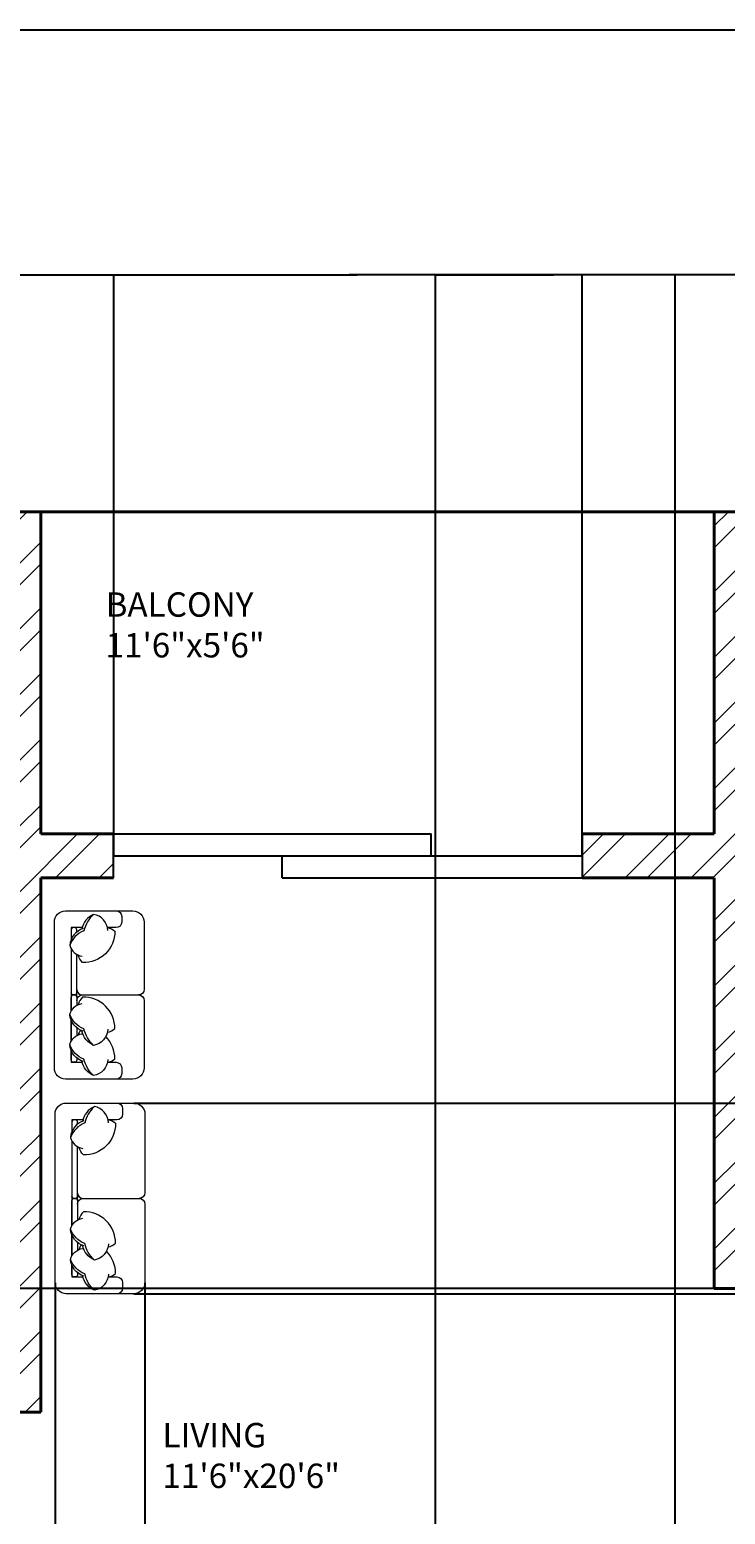
# Model space of a CAD drawing. Units: inches. Extents: x 1601 to 2297, y 1496 to 2631.
# Tile 51 of 57: x 1891 to 2033, y 2327 to 2631. Entities that reach past the tile are written whole.
import ezdxf

# ---------------------------------------------------------------- set-up
doc = ezdxf.new("R2010")
doc.units = ezdxf.units.IN
for name, color, linetype, lineweight in [('A-ANNO-DIMS', 2, 'Continuous', 18), ('A-ANNO-TTLB', 7, 'Continuous', 25), ('A-AREA-IDEN', 7, 'Continuous', 18), ('A-DOOR', 21, 'Continuous', 25), ('A-FURN', 8, 'Continuous', 18), ('A-WALL', 7, 'Continuous', 40), ('A-WALL-PATT', 215, 'Continuous', 13)]:
    doc.layers.add(name, color=color, linetype=linetype, lineweight=lineweight)
doc.styles.get("Standard").update_dxf_attribs({"font": 'arial.ttf'})
doc.dimstyles.get("Standard").update_dxf_attribs({"dimtxt": 0.18, "dimasz": 0.18, "dimexe": 0.18, "dimexo": 0.0625, "dimgap": 0.09, "dimtad": 0, "dimtih": 1, "dimtoh": 1, "dimdec": 4, "dimzin": 0, "dimdsep": 46, "dimtxsty": 'Standard', "dimcen": 0.09, "dimadec": 0, "dimazin": 0, "dimtfac": 1, "dimtdec": 4, "dimtofl": 0, "dimtmove": 0, "dimatfit": 3, "dimfxl": 1, "dimtolj": 1, "dimtzin": 0, "dimarcsym": 0})

# ---------------------------------------------------------------- blocks, each defined once
blk = doc.blocks.new('*D28')
at = {"layer": 'A-ANNO-DIMS', "color": 0, "lineweight": -2, "transparency": 16777216}
for p, q in [((1686.04, 2532.39), (1686.04, 2581.06)), ((1686.22, 2580.88), (1957.89, 2580.88)), ((2230.36, 2580.88), (1958.68, 2580.88)), ((2230.54, 2532.39), (2230.54, 2581.06))]:
    blk.add_line(p, q, dxfattribs=at)
at = {"layer": 'A-ANNO-DIMS', "color": 0, "transparency": 16777216}
for points in [[(1686.22, 2580.91), (1686.22, 2580.85), (1686.04, 2580.88)], [(2230.36, 2580.91), (2230.36, 2580.85), (2230.54, 2580.88)]]:
    blk.add_solid(points, dxfattribs=at)
at = {"layer": 'Defpoints', "color": 0, "transparency": 16777216}
for p in [(2230.54, 2580.88), (1686.04, 2532.33), (2230.54, 2532.33)]:
    blk.add_point(p, dxfattribs=at)
at = {"layer": 'A-ANNO-DIMS', "color": 0, "transparency": 16777216, "insert": (1958.29, 2580.88), "char_height": 0.18, "attachment_point": 5}
blk.add_mtext('\\A1;544.5', dxfattribs=at)
blk = doc.blocks.new('*D47')
at = {"layer": 'A-ANNO-DIMS', "color": 0, "lineweight": -2, "transparency": 16777216}
for p, q in [((1973.94, 2211.39), (1973.94, 2581.06)), ((1974.12, 2580.88), (1998.07, 2580.88)), ((2022.83, 2580.88), (1998.87, 2580.88)), ((2023.01, 2211.39), (2023.01, 2581.06))]:
    blk.add_line(p, q, dxfattribs=at)
at = {"layer": 'A-ANNO-DIMS', "color": 0, "transparency": 16777216}
for points in [[(1974.12, 2580.91), (1974.12, 2580.85), (1973.94, 2580.88)], [(2022.83, 2580.91), (2022.83, 2580.85), (2023.01, 2580.88)]]:
    blk.add_solid(points, dxfattribs=at)
at = {"layer": 'Defpoints', "color": 0, "transparency": 16777216}
for p in [(2023.01, 2580.88), (1973.94, 2211.33), (2023.01, 2211.33)]:
    blk.add_point(p, dxfattribs=at)
at = {"layer": 'A-ANNO-DIMS', "color": 0, "transparency": 16777216, "insert": (1998.47, 2580.88), "char_height": 0.18, "attachment_point": 5}
blk.add_mtext('\\A1;49.07', dxfattribs=at)
blk = doc.blocks.new('*D48')
at = {"layer": 'A-ANNO-DIMS', "color": 0, "lineweight": -2, "transparency": 16777216}
for p, q in [((2030.97, 2373.19), (1637.31, 2373.19)), ((1637.49, 2373.01), (1637.49, 2336.69)), ((1637.49, 2300.01), (1637.49, 2336.33)), ((2030.97, 2299.83), (1637.31, 2299.83))]:
    blk.add_line(p, q, dxfattribs=at)
at = {"layer": 'A-ANNO-DIMS', "color": 0, "transparency": 16777216}
for points in [[(1637.46, 2373.01), (1637.52, 2373.01), (1637.49, 2373.19)], [(1637.46, 2300.01), (1637.52, 2300.01), (1637.49, 2299.83)]]:
    blk.add_solid(points, dxfattribs=at)
at = {"layer": 'Defpoints', "color": 0, "transparency": 16777216}
for p in [(1637.49, 2373.19), (2031.04, 2373.19), (2031.04, 2299.83)]:
    blk.add_point(p, dxfattribs=at)
at = {"layer": 'A-ANNO-DIMS', "color": 0, "transparency": 16777216, "insert": (1637.49, 2336.51), "char_height": 0.18, "attachment_point": 5}
blk.add_mtext('\\A1;73.37', dxfattribs=at)
blk = doc.blocks.new('*D49')
at = {"layer": 'A-ANNO-DIMS', "color": 0, "lineweight": -2, "transparency": 16777216}
for p, q in [((1907.99, 2466.39), (1907.99, 2581.06)), ((1908.17, 2580.88), (1955.77, 2580.88)), ((2003.81, 2580.88), (1956.21, 2580.88)), ((2003.99, 2466.39), (2003.99, 2581.06))]:
    blk.add_line(p, q, dxfattribs=at)
at = {"layer": 'A-ANNO-DIMS', "color": 0, "transparency": 16777216}
for points in [[(1908.17, 2580.91), (1908.17, 2580.85), (1907.99, 2580.88)], [(2003.81, 2580.91), (2003.81, 2580.85), (2003.99, 2580.88)]]:
    blk.add_solid(points, dxfattribs=at)
at = {"layer": 'Defpoints', "color": 0, "transparency": 16777216}
for p in [(2003.99, 2580.88), (1907.99, 2466.33), (2003.99, 2466.33)]:
    blk.add_point(p, dxfattribs=at)
at = {"layer": 'A-ANNO-DIMS', "color": 0, "transparency": 16777216, "insert": (1955.99, 2580.88), "char_height": 0.18, "attachment_point": 5}
blk.add_mtext('\\A1;96', dxfattribs=at)
blk = doc.blocks.new('*D50')
at = {"layer": 'A-ANNO-DIMS', "color": 0, "lineweight": -2, "transparency": 16777216}
for p, q in [((1895.99, 2374.33), (1895.99, 1513.75)), ((1914.39, 2374.33), (1914.39, 1513.75)), ((1896.17, 1513.93), (1904.87, 1513.93)), ((1914.21, 1513.93), (1905.5, 1513.93))]:
    blk.add_line(p, q, dxfattribs=at)
at = {"layer": 'A-ANNO-DIMS', "color": 0, "transparency": 16777216}
for points in [[(1896.17, 1513.96), (1896.17, 1513.9), (1895.99, 1513.93)], [(1914.21, 1513.96), (1914.21, 1513.9), (1914.39, 1513.93)]]:
    blk.add_solid(points, dxfattribs=at)
at = {"layer": 'Defpoints', "color": 0, "transparency": 16777216}
for p in [(1895.99, 2374.4), (1914.39, 2374.4), (1914.39, 1513.93)]:
    blk.add_point(p, dxfattribs=at)
at = {"layer": 'A-ANNO-DIMS', "color": 0, "transparency": 16777216, "insert": (1905.19, 1513.93), "char_height": 0.18, "attachment_point": 5}
blk.add_mtext('\\A1;18.4', dxfattribs=at)
blk = doc.blocks.new('*D51')
at = {"layer": 'A-ANNO-DIMS', "color": 0, "lineweight": -2, "transparency": 16777216}
for p, q in [((1912.15, 2411.19), (2279.27, 2411.19)), ((2279.09, 2411.01), (2279.09, 2391.83)), ((2279.09, 2372.28), (2279.09, 2391.46)), ((1912.15, 2372.1), (2279.27, 2372.1))]:
    blk.add_line(p, q, dxfattribs=at)
at = {"layer": 'A-ANNO-DIMS', "color": 0, "transparency": 16777216}
for points in [[(2279.06, 2411.01), (2279.12, 2411.01), (2279.09, 2411.19)], [(2279.06, 2372.28), (2279.12, 2372.28), (2279.09, 2372.1)]]:
    blk.add_solid(points, dxfattribs=at)
at = {"layer": 'Defpoints', "color": 0, "transparency": 16777216}
for p in [(1912.09, 2411.19), (2279.09, 2411.19), (1912.09, 2372.1)]:
    blk.add_point(p, dxfattribs=at)
at = {"layer": 'A-ANNO-DIMS', "color": 0, "transparency": 16777216, "insert": (2279.09, 2391.64), "char_height": 0.18, "attachment_point": 5}
blk.add_mtext('\\A1;39.1', dxfattribs=at)

msp = doc.modelspace()

# ---------------------------------------------------------------- hatches: boundary and pattern name
at = {"layer": 'A-WALL-PATT'}
h = msp.add_hatch(dxfattribs=at)
h.set_pattern_fill('ANSI32', color=256)
h.paths.add_polyline_path([(1842.0336, 2528.0767), (1842.0336, 2532.3254), (1686.0373, 2532.3254), (1686.0373, 2492.9493), (1695.0373, 2492.9493), (1695.0373, 2523.3254), (1827.0373, 2523.3254), (1827.0373, 2416.8254), (1834.6225, 2416.8254), (1834.6225, 2419.0754), (1834.6225, 2421.3254), (1831.5373, 2421.3254), (1831.5373, 2523.3254), (1842.0336, 2523.3254)])
h.paths.add_polyline_path([(1695.0373, 2432.9493), (1686.0373, 2432.9493), (1686.0373, 2325.989), (1695.0373, 2325.989), (1695.0373, 2347.8254), (1827.0373, 2347.8254), (1827.0373, 2287.8254), (1823.2991, 2287.8254), (1823.2991, 2283.3254), (1847.9422, 2283.3254), (1847.9422, 2285.5754), (1847.9422, 2287.8254), (1831.5373, 2287.8254), (1831.5373, 2347.8254), (1846.9946, 2347.8254), (1846.9946, 2350.0754), (1846.9946, 2352.3254), (1695.0373, 2352.3254)])
h.paths.add_polyline_path([(1807.1169, 1573.5395), (2055.0405, 1573.5395), (2055.0405, 1610.6322), (1807.1169, 1610.6322)], flags=9)
h.paths.add_polyline_path([(1841.1631, 1712.7967), (1870.3957, 1712.7967), (1870.3957, 1731.454), (1841.1631, 1731.454)], flags=9)
h.paths.add_polyline_path([(2144.3862, 1772.185), (2191.0233, 1772.185), (2191.0233, 1790.8423), (2144.3862, 1790.8423)], flags=9)
h.paths.add_polyline_path([(2143.0128, 1827.3312), (2177.9958, 1827.3312), (2177.9958, 1845.9886), (2143.0128, 1845.9886)], flags=9)
h.paths.add_polyline_path([(2041.2439, 1833.5691), (2070.8516, 1833.5691), (2070.8516, 1852.2264), (2041.2439, 1852.2264)], flags=9)
h.paths.add_polyline_path([(2097.2791, 1947.0598), (2134.2061, 1947.0598), (2134.2061, 1965.7171), (2097.2791, 1965.7171)], flags=9)
h.paths.add_polyline_path([(2214.995, 1904.3124), (2214.995, 1942.2899), (2196.3376, 1942.2899), (2196.3376, 1904.3124)], flags=9)
h.paths.add_polyline_path([(2186.6284, 2043.8031), (2219.7935, 2043.8031), (2219.7935, 2062.4605), (2186.6284, 2062.4605)], flags=9)
h.paths.add_polyline_path([(2064.0877, 2031.616), (2097.4949, 2031.616), (2097.4949, 2050.2734), (2064.0877, 2050.2734)], flags=9)
h.paths.add_polyline_path([(1973.1349, 1986.0688), (2008.4009, 1986.0688), (2008.4009, 2004.7261), (1973.1349, 2004.7261)], flags=9)
h.paths.add_polyline_path([(1976.3676, 2106.9635), (2005.7469, 2106.9635), (2005.7469, 2125.6209), (1976.3676, 2125.6209)], flags=9)
h.paths.add_polyline_path([(1991.7852, 2180.4863), (2027.0513, 2180.4863), (2027.0513, 2199.1437), (1991.7852, 2199.1437)], flags=9)
h.paths.add_polyline_path([(2106.1801, 2187.9359), (2152.2101, 2187.9359), (2152.2101, 2206.5932), (2106.1801, 2206.5932)], flags=9)
h.paths.add_polyline_path([(2148.6686, 2262.2542), (2182.318, 2262.2542), (2182.318, 2280.9115), (2148.6686, 2280.9115)], flags=9)
h.paths.add_polyline_path([(2041.6327, 2252.8147), (2071.2405, 2252.8147), (2071.2405, 2271.4721), (2041.6327, 2271.4721)], flags=9)
h.paths.add_polyline_path([(2063.9734, 2375.4265), (2100.9004, 2375.4265), (2100.9004, 2394.0839), (2063.9734, 2394.0839)], flags=9)
h.paths.add_polyline_path([(2216.4955, 2330.9748), (2216.4955, 2370.2654), (2197.8381, 2370.2654), (2197.8381, 2330.9748)], flags=9)
h.paths.add_polyline_path([(2179.1416, 2485.8687), (2212.3067, 2485.8687), (2212.3067, 2504.5261), (2179.1416, 2504.5261)], flags=9)
h.paths.add_polyline_path([(2078.7442, 2471.1516), (2112.1514, 2471.1516), (2112.1514, 2489.809), (2078.7442, 2489.809)], flags=9)
h.paths.add_polyline_path([(1915.9631, 2329.4668), (1952.8902, 2329.4668), (1952.8902, 2348.1241), (1915.9631, 2348.1241)], flags=9)
h.paths.add_polyline_path([(1904.3189, 2499.6709), (1940.4512, 2499.6709), (1940.4512, 2518.3282), (1904.3189, 2518.3282)], flags=9)
h.paths.add_polyline_path([(1892.3665, 2100.4595), (1925.6374, 2100.4595), (1925.6374, 2119.1169), (1892.3665, 2119.1169)], flags=9)
h.paths.add_polyline_path([(1909.2984, 1805.9631), (1946.2254, 1805.9631), (1946.2254, 1824.6205), (1909.2984, 1824.6205)], flags=9)
h.paths.add_polyline_path([(1934.6056, 1658.616), (1970.738, 1658.616), (1970.738, 1677.2733), (1934.6056, 1677.2733)], flags=9)
h.paths.add_polyline_path([(1711.2052, 1789.8902), (1750.0456, 1789.8902), (1750.0456, 1808.5476), (1711.2052, 1808.5476)], flags=9)
h.paths.add_polyline_path([(1742.7874, 1854.6743), (1771.9449, 1854.6743), (1771.9449, 1873.3317), (1742.7874, 1873.3317)], flags=9)
h.paths.add_polyline_path([(1807.3592, 1997.7912), (1850.1116, 1997.7912), (1850.1116, 2016.4486), (1807.3592, 2016.4486)], flags=9)
h.paths.add_polyline_path([(1717.4579, 2237.7844), (1760.2103, 2237.7844), (1760.2103, 2256.4417), (1717.4579, 2256.4417)], flags=9)
h.paths.add_polyline_path([(1780.9285, 2324.0623), (1810.086, 2324.0623), (1810.086, 2342.7197), (1780.9285, 2342.7197)], flags=25)
h.paths.add_polyline_path([(1837.696, 2449.2024), (1866.9286, 2449.2024), (1866.9286, 2467.8598), (1837.696, 2467.8598)], flags=9)
h.paths.add_polyline_path([(1712.7752, 2484.9404), (1751.6156, 2484.9404), (1751.6156, 2503.5977), (1712.7752, 2503.5977)], flags=25)
h = msp.add_hatch(dxfattribs=at)
h.set_pattern_fill('ANSI32', color=256)
h.paths.add_polyline_path([(2230.5373, 2532.3254), (2106.0595, 2532.3254), (2106.0595, 2523.3254), (2169.0373, 2523.3254), (2169.0373, 2424.3254), (2091.3989, 2424.3254), (2091.3989, 2419.8254), (2169.0373, 2419.8254), (2169.0373, 2408.1385), (2178.0373, 2408.1385), (2178.0373, 2419.8254), (2181.0581, 2419.8254), (2181.0581, 2422.0754), (2181.0581, 2424.3254), (2178.0373, 2424.3254), (2178.0373, 2523.3254), (2226.0373, 2523.3254), (2226.0373, 2424.3254), (2206.6251, 2424.3254), (2206.6251, 2419.8254), (2226.0373, 2419.8254), (2226.0373, 2299.8254), (2226.0373, 2295.3254), (2178.0373, 2295.3254), (2178.0373, 2312.1385), (2169.0373, 2312.1385), (2169.0373, 2295.3254), (2130.0373, 2295.3254), (2130.0373, 2279.1364), (2128.0593, 2279.1364), (2128.0593, 2274.6364), (2130.0373, 2274.6364), (2130.0373, 2260.7505), (2134.5373, 2260.7505), (2134.5373, 2290.8254), (2226.0373, 2290.8254), (2226.0373, 2279.2475), (2230.5373, 2279.2475), (2230.5373, 2347.8254)])
h.paths.add_polyline_path([(2070.0595, 2532.3254), (2031.0373, 2532.3254), (2031.0373, 2466.3254), (2003.9878, 2466.3254), (2003.9878, 2457.3254), (2031.0373, 2457.3254), (2031.0373, 2419.8254), (2031.0373, 2373.1914), (2035.5373, 2373.1914), (2035.5373, 2419.8254), (2047.3393, 2419.8254), (2047.3393, 2424.3254), (2035.5373, 2424.3254), (2035.5373, 2523.3254), (2070.0595, 2523.3254), (2070.0595, 2527.8254)])
h.paths.add_polyline_path([(1893.0373, 2532.3254), (1866.0336, 2532.3254), (1866.0336, 2523.3254), (1888.5373, 2523.3254), (1888.5373, 2347.8254), (1893.0373, 2347.8254), (1893.0373, 2457.3254), (1907.9878, 2457.3254), (1907.9878, 2466.3254), (1893.0373, 2466.3254)])
h = msp.add_hatch(dxfattribs=at)
h.set_pattern_fill('ANSI32', color=256)
h.paths.add_polyline_path([(1973.9371, 2211.3254), (1893.0373, 2211.3254), (1893.0373, 2287.8254), (1884.6167, 2287.8254), (1884.6167, 2285.5754), (1884.6167, 2283.3254), (1888.5373, 2283.3254), (1888.5373, 2145.3254), (1695.0373, 2145.3254), (1695.0373, 2173.8724), (1690.5373, 2173.8724), (1686.0373, 2173.8724), (1686.0373, 2136.3254), (1722.5687, 2136.3254), (1722.5687, 2117.4352), (1731.5687, 2117.4352), (1731.5687, 2136.3254), (1893.0373, 2136.3254), (1893.0373, 2202.3254), (1959.0373, 2202.3254), (1959.0373, 2182.1303), (1968.0373, 2182.1303), (1968.0373, 2202.3254), (1973.9371, 2202.3254)])
h.paths.add_polyline_path([(2094.0373, 2274.6364), (2096.4294, 2274.6364), (2096.4294, 2276.8864), (2096.4294, 2279.1364), (2094.0373, 2279.1364), (2094.0373, 2290.8254), (2094.0373, 2295.3254), (2089.5373, 2295.3254), (2089.5373, 2230.8254), (2035.5373, 2230.8254), (2035.5373, 2299.8254), (2031.0373, 2299.8254), (2031.0373, 2211.3254), (2023.0065, 2211.3254), (2023.0065, 2202.3254), (2031.0373, 2202.3254), (2031.0373, 2140.8254), (1968.0373, 2140.8254), (1968.0373, 2145.9106), (1963.5373, 2145.9106), (1959.0373, 2145.9106), (1959.0373, 2116.839), (1963.5373, 2116.839), (1968.0373, 2116.839), (1968.0373, 2131.8254), (2031.0373, 2131.8254), (2031.0373, 2094.3254), (2031.0373, 2085.3254), (2031.0373, 2056.8254), (1968.0373, 2056.8254), (1968.0373, 2070.4947), (1963.5373, 2070.4947), (1959.0373, 2070.4947), (1959.0373, 2040.3029), (1968.0373, 2040.3029), (1968.0373, 2047.8254), (2031.0373, 2047.8254), (2031.0373, 1983.3254), (2031.0373, 1978.8254), (2021.1979, 1978.8254), (2021.1979, 1974.3254), (2031.0373, 1974.3254), (2031.0373, 1954.3528), (2035.5373, 1954.3528), (2035.5373, 1974.3254), (2035.5373, 1981.8254), (2055.5513, 1981.8254), (2055.5513, 1986.3254), (2035.5373, 1986.3254), (2035.5373, 2047.8254), (2040.0373, 2047.8254), (2040.0373, 2085.3254), (2040.0373, 2094.3254), (2040.0373, 2140.8254), (2035.5373, 2140.8254), (2035.5373, 2226.3254), (2089.5373, 2226.3254), (2094.0373, 2226.3254)])
h.paths.add_polyline_path([(2226.0373, 2230.8254), (2134.5373, 2230.8254), (2134.5373, 2233.5437), (2130.0373, 2233.5437), (2130.0373, 2226.3254), (2134.5373, 2226.3254), (2226.0373, 2226.3254)])
h.paths.add_polyline_path([(1807.1169, 1573.5395), (2055.0405, 1573.5395), (2055.0405, 1610.6322), (1807.1169, 1610.6322)], flags=9)
h.paths.add_polyline_path([(1841.1631, 1712.7967), (1870.3957, 1712.7967), (1870.3957, 1731.454), (1841.1631, 1731.454)], flags=9)
h.paths.add_polyline_path([(2144.3862, 1772.185), (2191.0233, 1772.185), (2191.0233, 1790.8423), (2144.3862, 1790.8423)], flags=9)
h.paths.add_polyline_path([(2143.0128, 1827.3312), (2177.9958, 1827.3312), (2177.9958, 1845.9886), (2143.0128, 1845.9886)], flags=9)
h.paths.add_polyline_path([(2041.2439, 1833.5691), (2070.8516, 1833.5691), (2070.8516, 1852.2264), (2041.2439, 1852.2264)], flags=9)
h.paths.add_polyline_path([(2097.2791, 1947.0598), (2134.2061, 1947.0598), (2134.2061, 1965.7171), (2097.2791, 1965.7171)], flags=9)
h.paths.add_polyline_path([(2214.995, 1904.3124), (2214.995, 1942.2899), (2196.3376, 1942.2899), (2196.3376, 1904.3124)], flags=9)
h.paths.add_polyline_path([(2186.6284, 2043.8031), (2219.7935, 2043.8031), (2219.7935, 2062.4605), (2186.6284, 2062.4605)], flags=9)
h.paths.add_polyline_path([(2064.0877, 2031.616), (2097.4949, 2031.616), (2097.4949, 2050.2734), (2064.0877, 2050.2734)], flags=9)
h.paths.add_polyline_path([(1973.1349, 1986.0688), (2008.4009, 1986.0688), (2008.4009, 2004.7261), (1973.1349, 2004.7261)], flags=25)
h.paths.add_polyline_path([(1976.3676, 2106.9635), (2005.7469, 2106.9635), (2005.7469, 2125.6209), (1976.3676, 2125.6209)], flags=25)
h.paths.add_polyline_path([(1991.7852, 2180.4863), (2027.0513, 2180.4863), (2027.0513, 2199.1437), (1991.7852, 2199.1437)], flags=25)
h.paths.add_polyline_path([(2106.1801, 2187.9359), (2152.2101, 2187.9359), (2152.2101, 2206.5932), (2106.1801, 2206.5932)], flags=9)
h.paths.add_polyline_path([(2148.6686, 2262.2542), (2182.318, 2262.2542), (2182.318, 2280.9115), (2148.6686, 2280.9115)], flags=9)
h.paths.add_polyline_path([(2041.6327, 2252.8147), (2071.2405, 2252.8147), (2071.2405, 2271.4721), (2041.6327, 2271.4721)], flags=25)
h.paths.add_polyline_path([(2063.9734, 2375.4265), (2100.9004, 2375.4265), (2100.9004, 2394.0839), (2063.9734, 2394.0839)], flags=9)
h.paths.add_polyline_path([(2216.4955, 2330.9748), (2216.4955, 2370.2654), (2197.8381, 2370.2654), (2197.8381, 2330.9748)], flags=9)
h.paths.add_polyline_path([(2179.1416, 2485.8687), (2212.3067, 2485.8687), (2212.3067, 2504.5261), (2179.1416, 2504.5261)], flags=9)
h.paths.add_polyline_path([(2078.7442, 2471.1516), (2112.1514, 2471.1516), (2112.1514, 2489.809), (2078.7442, 2489.809)], flags=9)
h.paths.add_polyline_path([(1915.9631, 2329.4668), (1952.8902, 2329.4668), (1952.8902, 2348.1241), (1915.9631, 2348.1241)], flags=9)
h.paths.add_polyline_path([(1904.3189, 2499.6709), (1940.4512, 2499.6709), (1940.4512, 2518.3282), (1904.3189, 2518.3282)], flags=9)
h.paths.add_polyline_path([(1892.3665, 2100.4595), (1925.6374, 2100.4595), (1925.6374, 2119.1169), (1892.3665, 2119.1169)], flags=9)
h.paths.add_polyline_path([(1909.2984, 1805.9631), (1946.2254, 1805.9631), (1946.2254, 1824.6205), (1909.2984, 1824.6205)], flags=9)
h.paths.add_polyline_path([(1934.6056, 1658.616), (1970.738, 1658.616), (1970.738, 1677.2733), (1934.6056, 1677.2733)], flags=9)
h.paths.add_polyline_path([(1711.2052, 1789.8902), (1750.0456, 1789.8902), (1750.0456, 1808.5476), (1711.2052, 1808.5476)], flags=9)
h.paths.add_polyline_path([(1742.7874, 1854.6743), (1771.9449, 1854.6743), (1771.9449, 1873.3317), (1742.7874, 1873.3317)], flags=9)
h.paths.add_polyline_path([(1807.3592, 1997.7912), (1850.1116, 1997.7912), (1850.1116, 2016.4486), (1807.3592, 2016.4486)], flags=9)
h.paths.add_polyline_path([(1717.4579, 2237.7844), (1760.2103, 2237.7844), (1760.2103, 2256.4417), (1717.4579, 2256.4417)], flags=25)
h.paths.add_polyline_path([(1780.9285, 2324.0623), (1810.086, 2324.0623), (1810.086, 2342.7197), (1780.9285, 2342.7197)], flags=9)
h.paths.add_polyline_path([(1837.696, 2449.2024), (1866.9286, 2449.2024), (1866.9286, 2467.8598), (1837.696, 2467.8598)], flags=9)
h.paths.add_polyline_path([(1712.7752, 2484.9404), (1751.6156, 2484.9404), (1751.6156, 2503.5977), (1712.7752, 2503.5977)], flags=9)
h = msp.add_hatch(dxfattribs=at)
h.set_pattern_fill('ANSI32', color=256)
h.paths.add_polyline_path([(2230.5373, 1861.8254), (2182.5373, 1861.8254), (2182.5373, 1885.3637), (2178.0373, 1885.3637), (2178.0373, 1861.8254), (2166.0373, 1861.8254), (2134.5373, 1861.8254), (2130.0373, 1861.8254), (2130.0373, 1841.4682), (2126.8833, 1841.4682), (2126.8833, 1836.9682), (2130.0373, 1836.9682), (2130.0373, 1822.7302), (2134.5373, 1822.7302), (2134.5373, 1857.3254), (2166.0373, 1857.3254), (2226.0373, 1857.3254), (2226.0373, 1846.1155), (2230.5373, 1846.1155)])
h.paths.add_polyline_path([(2226.0373, 1797.3254), (2134.5373, 1797.3254), (2134.5373, 1800.6636), (2132.2873, 1800.6636), (2130.0373, 1800.6636), (2130.0373, 1797.3254), (2130.0373, 1792.8254), (2167.7264, 1792.8254), (2226.0373, 1792.8254)])
h.paths.add_polyline_path([(2230.5373, 1822.1155), (2226.0373, 1822.1155), (2226.0373, 1760.8563), (2230.5373, 1760.8563)])
h.paths.add_polyline_path([(2230.5373, 1700.8563), (2226.0373, 1700.8563), (2226.0373, 1644.3254), (2140.2517, 1644.3254), (2140.2517, 1635.3254), (2230.5373, 1635.3254)])
h.paths.add_polyline_path([(2080.2517, 1639.8254), (2080.2517, 1644.3254), (2035.5373, 1644.3254), (2035.5373, 1792.8254), (2094.0373, 1792.8254), (2094.0373, 1797.3254), (2094.0373, 1836.9682), (2097.1057, 1836.9682), (2097.1057, 1839.2182), (2097.1057, 1841.4682), (2094.0373, 1841.4682), (2094.0373, 1862.2276), (2089.5373, 1862.2276), (2089.5373, 1797.3254), (2035.5373, 1797.3254), (2035.5373, 1857.3254), (2035.5373, 1885.0916), (2031.0373, 1885.0916), (2031.0373, 1710.3254), (2012.329, 1710.3254), (2012.329, 1701.3254), (2031.0373, 1701.3254), (2031.0373, 1644.3254), (2031.0373, 1635.3254), (2080.2517, 1635.3254)])
h.paths.add_polyline_path([(1836.0373, 1653.2033), (1842.6171, 1653.2033), (1842.6171, 1657.7033), (1842.6171, 1662.2033), (1831.5373, 1662.2033), (1831.5373, 1764.2033), (1835.3881, 1764.2033), (1835.3881, 1766.4533), (1835.3881, 1768.7033), (1831.5373, 1768.7033), (1827.0373, 1768.7033), (1827.0373, 1662.2033), (1827.0373, 1635.3254), (1836.0373, 1635.3254)])
h.paths.add_polyline_path([(1893.0373, 1701.3254), (1907.193, 1701.3254), (1907.193, 1705.8254), (1907.193, 1710.3254), (1893.0373, 1710.3254), (1893.0373, 1819.8254), (1882.6444, 1819.8254), (1882.6444, 1817.5754), (1882.6444, 1815.3254), (1888.5373, 1815.3254), (1888.5373, 1662.2033), (1884.0373, 1662.2033), (1866.6171, 1662.2033), (1866.6171, 1653.2033), (1882.391, 1653.2033), (1884.0373, 1653.2033), (1884.0373, 1635.3254), (1893.0373, 1635.3254)])
h.paths.add_polyline_path([(1739.3335, 1639.8254), (1739.3335, 1644.3254), (1695.0373, 1644.3254), (1695.0373, 1702.0135), (1690.5373, 1702.0135), (1686.0373, 1702.0135), (1686.0373, 1635.3254), (1739.3335, 1635.3254)])
h.paths.add_polyline_path([(1827.0373, 1644.3254), (1799.3335, 1644.3254), (1799.3335, 1635.3254), (1827.0373, 1635.3254)])
h.paths.add_polyline_path([(1695.0373, 1815.3254), (1849.2759, 1815.3254), (1849.2759, 1819.8254), (1807.5373, 1819.8254), (1807.5373, 1879.8254), (1851.1533, 1879.8254), (1851.1533, 1882.0754), (1851.1533, 1884.3254), (1799.3405, 1884.3254), (1799.3405, 1882.0754), (1799.3405, 1879.8254), (1803.0373, 1879.8254), (1803.0373, 1819.8254), (1695.0373, 1819.8254), (1695.0373, 1835.0458), (1690.5373, 1835.0458), (1686.0373, 1835.0458), (1686.0373, 1766.1753), (1695.0373, 1766.1753)])
h.paths.add_polyline_path([(1775.8157, 1884.3254), (1695.0373, 1884.3254), (1695.0373, 1912.9526), (1690.5373, 1912.9526), (1686.0373, 1912.9526), (1686.0373, 1859.0458), (1695.0373, 1859.0458), (1695.0373, 1879.8254), (1775.8157, 1879.8254)])
h.paths.add_polyline_path([(1893.0373, 2031.3254), (1731.5687, 2031.3254), (1731.5687, 2057.4352), (1722.5687, 2057.4352), (1722.5687, 2031.3254), (1686.0373, 2031.3254), (1686.0373, 1972.9526), (1695.0373, 1972.9526), (1695.0373, 2022.3254), (1888.5373, 2022.3254), (1888.5373, 1884.3254), (1883.4996, 1884.3254), (1883.4996, 1879.8254), (1893.0373, 1879.8254), (1893.0373, 1974.3254), (1976.6199, 1974.3254), (1976.6199, 1978.8254), (1968.0373, 1978.8254), (1968.0373, 1983.3254), (1968.0373, 2008.4756), (1963.5373, 2008.4756), (1959.0373, 2008.4756), (1959.0373, 1983.3254), (1893.0373, 1983.3254)])
h.paths.add_polyline_path([(2230.5373, 2140.4745), (2226.0373, 2140.4745), (2226.0373, 2094.3254), (2040.0373, 2094.3254), (2040.0373, 2085.3254), (2178.0373, 2085.3254), (2178.0373, 2065.6965), (2182.5373, 2065.6965), (2182.5373, 2085.3254), (2226.0373, 2085.3254), (2226.0373, 1986.3254), (2211.2679, 1986.3254), (2211.2679, 1981.8254), (2230.5373, 1981.8254)])
h.paths.add_polyline_path([(2187.6292, 1986.3254), (2182.5373, 1986.3254), (2182.5373, 2029.6965), (2178.0373, 2029.6965), (2178.0373, 1986.3254), (2099.05, 1986.3254), (2099.05, 1981.8254), (2178.0373, 1981.8254), (2178.0373, 1969.3637), (2182.5373, 1969.3637), (2182.5373, 1981.8254), (2187.6292, 1981.8254), (2187.6292, 1984.0754)])
h.paths.add_polyline_path([(1807.1169, 1573.5395), (2055.0405, 1573.5395), (2055.0405, 1610.6322), (1807.1169, 1610.6322)], flags=9)
h.paths.add_polyline_path([(1841.1631, 1712.7967), (1870.3957, 1712.7967), (1870.3957, 1731.454), (1841.1631, 1731.454)], flags=9)
h.paths.add_polyline_path([(2144.3862, 1772.185), (2191.0233, 1772.185), (2191.0233, 1790.8423), (2144.3862, 1790.8423)], flags=9)
h.paths.add_polyline_path([(2143.0128, 1827.3312), (2177.9958, 1827.3312), (2177.9958, 1845.9886), (2143.0128, 1845.9886)], flags=25)
h.paths.add_polyline_path([(2041.2439, 1833.5691), (2070.8516, 1833.5691), (2070.8516, 1852.2264), (2041.2439, 1852.2264)], flags=25)
h.paths.add_polyline_path([(2097.2791, 1947.0598), (2134.2061, 1947.0598), (2134.2061, 1965.7171), (2097.2791, 1965.7171)], flags=9)
h.paths.add_polyline_path([(2214.995, 1904.3124), (2214.995, 1942.2899), (2196.3376, 1942.2899), (2196.3376, 1904.3124)], flags=9)
h.paths.add_polyline_path([(2186.6284, 2043.8031), (2219.7935, 2043.8031), (2219.7935, 2062.4605), (2186.6284, 2062.4605)], flags=25)
h.paths.add_polyline_path([(2064.0877, 2031.616), (2097.4949, 2031.616), (2097.4949, 2050.2734), (2064.0877, 2050.2734)], flags=25)
h.paths.add_polyline_path([(1973.1349, 1986.0688), (2008.4009, 1986.0688), (2008.4009, 2004.7261), (1973.1349, 2004.7261)], flags=9)
h.paths.add_polyline_path([(1976.3676, 2106.9635), (2005.7469, 2106.9635), (2005.7469, 2125.6209), (1976.3676, 2125.6209)], flags=9)
h.paths.add_polyline_path([(1991.7852, 2180.4863), (2027.0513, 2180.4863), (2027.0513, 2199.1437), (1991.7852, 2199.1437)], flags=9)
h.paths.add_polyline_path([(2106.1801, 2187.9359), (2152.2101, 2187.9359), (2152.2101, 2206.5932), (2106.1801, 2206.5932)], flags=9)
h.paths.add_polyline_path([(2148.6686, 2262.2542), (2182.318, 2262.2542), (2182.318, 2280.9115), (2148.6686, 2280.9115)], flags=9)
h.paths.add_polyline_path([(2041.6327, 2252.8147), (2071.2405, 2252.8147), (2071.2405, 2271.4721), (2041.6327, 2271.4721)], flags=9)
h.paths.add_polyline_path([(2063.9734, 2375.4265), (2100.9004, 2375.4265), (2100.9004, 2394.0839), (2063.9734, 2394.0839)], flags=9)
h.paths.add_polyline_path([(2216.4955, 2330.9748), (2216.4955, 2370.2654), (2197.8381, 2370.2654), (2197.8381, 2330.9748)], flags=9)
h.paths.add_polyline_path([(2179.1416, 2485.8687), (2212.3067, 2485.8687), (2212.3067, 2504.5261), (2179.1416, 2504.5261)], flags=9)
h.paths.add_polyline_path([(2078.7442, 2471.1516), (2112.1514, 2471.1516), (2112.1514, 2489.809), (2078.7442, 2489.809)], flags=9)
h.paths.add_polyline_path([(1915.9631, 2329.4668), (1952.8902, 2329.4668), (1952.8902, 2348.1241), (1915.9631, 2348.1241)], flags=9)
h.paths.add_polyline_path([(1904.3189, 2499.6709), (1940.4512, 2499.6709), (1940.4512, 2518.3282), (1904.3189, 2518.3282)], flags=9)
h.paths.add_polyline_path([(1892.3665, 2100.4595), (1925.6374, 2100.4595), (1925.6374, 2119.1169), (1892.3665, 2119.1169)], flags=9)
h.paths.add_polyline_path([(1909.2984, 1805.9631), (1946.2254, 1805.9631), (1946.2254, 1824.6205), (1909.2984, 1824.6205)], flags=9)
h.paths.add_polyline_path([(1934.6056, 1658.616), (1970.738, 1658.616), (1970.738, 1677.2733), (1934.6056, 1677.2733)], flags=9)
h.paths.add_polyline_path([(1711.2052, 1789.8902), (1750.0456, 1789.8902), (1750.0456, 1808.5476), (1711.2052, 1808.5476)], flags=25)
h.paths.add_polyline_path([(1742.7874, 1854.6743), (1771.9449, 1854.6743), (1771.9449, 1873.3317), (1742.7874, 1873.3317)], flags=25)
h.paths.add_polyline_path([(1807.3592, 1997.7912), (1850.1116, 1997.7912), (1850.1116, 2016.4486), (1807.3592, 2016.4486)], flags=25)
h.paths.add_polyline_path([(1717.4579, 2237.7844), (1760.2103, 2237.7844), (1760.2103, 2256.4417), (1717.4579, 2256.4417)], flags=9)
h.paths.add_polyline_path([(1780.9285, 2324.0623), (1810.086, 2324.0623), (1810.086, 2342.7197), (1780.9285, 2342.7197)], flags=9)
h.paths.add_polyline_path([(1837.696, 2449.2024), (1866.9286, 2449.2024), (1866.9286, 2467.8598), (1837.696, 2467.8598)], flags=9)
h.paths.add_polyline_path([(1712.7752, 2484.9404), (1751.6156, 2484.9404), (1751.6156, 2503.5977), (1712.7752, 2503.5977)], flags=9)

# ---------------------------------------------------------------- linework, layer by layer
at = {"layer": 'A-ANNO-TTLB'}
msp.add_lwpolyline([(1600.5933, 2631.1477), (2297.129, 2631.1477), (2297.129, 1496.1026), (1600.5933, 1496.1026)], close=True, dxfattribs=at)
at = {"layer": 'A-DOOR'}
for p, q in [((1907.9878, 2457.3254), (1907.9878, 2466.3254)), ((1907.9878, 2466.3254), (1907.9878, 2461.8254)), ((1907.9878, 2466.3254), (1973.0558, 2466.3254)), ((1973.0558, 2461.8254), (1973.0558, 2466.3254)), ((2003.9878, 2461.8254), (2003.9878, 2466.3254)), ((2003.9878, 2466.3254), (2003.9878, 2457.3254)), ((1907.9878, 2461.8254), (1979.9878, 2461.8254)), ((1942.5084, 2457.3254), (1942.5084, 2461.8254)), ((1979.9878, 2461.8254), (2003.9878, 2461.8254)), ((1942.5084, 2457.3254), (2003.9878, 2457.3254))]:
    msp.add_line(p, q, dxfattribs=at)
at = {"layer": 'A-FURN', "ltscale": 0.03}
for points in [[(1914.235, 2434.4811, -0.41421356), (1913.0851, 2433.3312, -0.41421356), (1914.235, 2432.1812), (1914.235, 2418.3817, -0.41421356), (1911.9351, 2416.0818), (1898.1356, 2416.0818, -0.41421356), (1895.8357, 2418.3817), (1895.8357, 2448.2806, -0.41421356), (1898.1356, 2450.5805), (1911.9351, 2450.5805, -0.41421356), (1914.235, 2448.2806), (1914.235, 2434.4811, -0.41421356), (1913.0851, 2433.3312, -0.41421356), (1914.235, 2432.1812)], [(1914.3895, 2392.7946, -0.41421356), (1913.2396, 2391.6446, -0.41421356), (1914.3895, 2390.4947), (1914.3895, 2374.3952, -0.41421356), (1912.0896, 2372.0953), (1898.2901, 2372.0953, -0.41421356), (1895.9902, 2374.3952), (1895.9902, 2408.894, -0.41421356), (1898.2901, 2411.1939), (1912.0896, 2411.1939, -0.41421356), (1914.3895, 2408.894), (1914.3895, 2392.7946, -0.41421356), (1913.2396, 2391.6446, -0.41421356), (1914.3895, 2390.4947)]]:
    msp.add_lwpolyline(points, format="xyb", dxfattribs=at)
at = {"layer": 'A-FURN'}
for points in [[(1903.8745, 2449.8487, 0.14772988), (1901.8982, 2446.4877, 0.21334276), (1898.9996, 2443.5221, 0.17866181)], [(1906.7731, 2446.5536, 0.35677236), (1903.8745, 2449.8487, 0.24954205), (1901.4858, 2446.863, -9.61688035)], [(1908.4853, 2450.5805, -0.41421356), (1909.6352, 2449.4306), (1909.6352, 2448.2806, -0.41421356), (1908.4853, 2447.1307), (1906.7035, 2447.1307)], [(1901.7407, 2446.952, 0.30666349), (1898.9996, 2443.5221, 0.30632997), (1901.503, 2441.2814, -0.87284716)], [(1900.4355, 2446.2531), (1900.4355, 2446.6707, 0.41421356), (1899.9756, 2447.1307), (1899.7456, 2447.1307, 0.41421356), (1899.2856, 2446.6707)], [(1899.2856, 2446.6707), (1899.2856, 2444.7115, 0.41421356)], [(1906.703, 2447.1332, -0.16554063), (1908.2224, 2446.4218, -0.42598917), (1901.6347, 2439.9634, -0.12152332), (1900.7267, 2441.4965, 7.11546429)], [(1899.2856, 2442.7984), (1899.2856, 2433.7912, 0.41421356), (1899.7456, 2433.3312), (1899.9756, 2433.3312, 0.41421356), (1900.4355, 2433.7912), (1900.4355, 2441.6404, 0.41421356)], [(1900.4355, 2434.4811, 0.41421356), (1901.5855, 2433.3312)], [(1900.4355, 2434.4811, 0.41421356), (1901.5855, 2433.3312), (1913.0851, 2433.3312, 0.41421356)], [(1901.7407, 2425.9051, -0.30666349), (1898.9996, 2429.335, -0.30632997), (1901.503, 2431.5757, 0.87284716)], [(1899.2856, 2430.0588), (1899.2856, 2432.8712, -0.41421356), (1899.7456, 2433.3312), (1899.9756, 2433.3312, -0.41421356), (1900.4355, 2432.8712), (1900.4355, 2431.2167, -0.41421356)], [(1900.4355, 2432.1812, -0.41421356), (1901.5855, 2433.3312)], [(1900.4355, 2432.1812, -0.41421356), (1901.5855, 2433.3312), (1913.0851, 2433.3312, -0.41421356)], [(1906.703, 2425.724, 0.16554063), (1908.2224, 2426.4354, 0.42598917), (1901.6347, 2432.8937, 0.12152332), (1900.7267, 2431.3606, -7.11546429)], [(1903.8745, 2423.0085, -0.14772988), (1901.8982, 2426.3695, -0.21334276), (1898.9996, 2429.335, -0.17866181)], [(1899.2856, 2423.864), (1899.2856, 2428.1456, -0.41421356)], [(1901.7407, 2419.7103, -0.30666349), (1898.9996, 2423.1403, -0.30632997), (1901.503, 2425.3809, 0.87284716)], [(1900.4355, 2426.604), (1900.4355, 2425.0219, -0.41421356)], [(1901.1763, 2426.13, 0.07186538), (1900.7267, 2425.1659, -7.11546429)], [(1906.7731, 2426.3036, -0.35677236), (1903.8745, 2423.0085, -0.24954205), (1901.4858, 2425.9941, 9.61688035)], [(1906.703, 2419.5292, 0.16554063), (1908.2224, 2420.2406, 0.20023115), (1906.3719, 2424.8055, 0.12152332)], [(1903.8745, 2416.8137, -0.14772988), (1901.8982, 2420.1747, -0.21334276), (1898.9996, 2423.1403, -0.17866181)], [(1899.2856, 2419.9917), (1899.2856, 2421.9509, -0.41421356)], [(1899.2856, 2421.9509), (1899.2856, 2419.5317), (1901.5455, 2419.5317, -0.41421356)], [(1900.4355, 2420.4092), (1900.4355, 2419.9917, -0.41421356), (1899.9756, 2419.5317), (1899.7456, 2419.5317, -0.41421356), (1899.2856, 2419.9917)], [(1906.7731, 2420.1088, -0.35677236), (1903.8745, 2416.8137, -0.24954205), (1901.4858, 2419.7993, 9.61688035)], [(1906.7035, 2419.5317), (1908.4853, 2419.5317, -0.41421356), (1909.6352, 2418.3817), (1909.6352, 2417.2318, -0.41421356), (1908.4853, 2416.0818)], [(1904.029, 2410.462, 0.14772988), (1902.0527, 2407.101, 0.21334276), (1899.1541, 2404.1354, 0.17866181)], [(1906.9276, 2407.1669, 0.35677236), (1904.029, 2410.462, 0.24954205), (1901.6403, 2407.4764, -9.61688035)], [(1908.6397, 2411.1939, -0.41421356), (1909.7897, 2410.0439), (1909.7897, 2408.894, -0.41421356), (1908.6397, 2407.744), (1906.858, 2407.744)], [(1901.8952, 2407.5653, 0.30666349), (1899.1541, 2404.1354, 0.30632997), (1901.6575, 2401.8948, -0.87284716)], [(1900.59, 2406.8665), (1900.59, 2407.284, 0.41421356), (1900.1301, 2407.744), (1899.9001, 2407.744, 0.41421356), (1899.4401, 2407.284)], [(1899.4401, 2407.284), (1899.4401, 2405.3248, 0.41421356)], [(1906.8575, 2407.7465, -0.16554063), (1908.3769, 2407.0351, -0.42598917), (1901.7892, 2400.5767, -0.12152332), (1900.8812, 2402.1098, 7.11546429)], [(1899.4401, 2403.4117), (1899.4401, 2392.1046, 0.41421356), (1899.9001, 2391.6446), (1900.1301, 2391.6446, 0.41421356), (1900.59, 2392.1046), (1900.59, 2402.2538, 0.41421356)], [(1899.4401, 2386.0723), (1899.4401, 2391.1846, -0.41421356), (1899.9001, 2391.6446), (1900.1301, 2391.6446, -0.41421356), (1900.59, 2391.1846), (1900.59, 2387.2302, -0.41421356)], [(1900.59, 2392.7946, 0.41421356), (1901.74, 2391.6446)], [(1900.59, 2392.7946, 0.41421356), (1901.74, 2391.6446), (1913.2396, 2391.6446, 0.41421356)], [(1900.59, 2390.4947, -0.41421356), (1901.74, 2391.6446)], [(1900.59, 2390.4947, -0.41421356), (1901.74, 2391.6446), (1913.2396, 2391.6446, -0.41421356)], [(1906.8575, 2381.7375, 0.16554063), (1908.3769, 2382.4489, 0.42598917), (1901.7892, 2388.9073, 0.12152332), (1900.8812, 2387.3742, -7.11546429)], [(1901.8952, 2381.9186, -0.30666349), (1899.1541, 2385.3486, -0.30632997), (1901.6575, 2387.5892, 0.87284716)], [(1904.029, 2379.022, -0.14772988), (1902.0527, 2382.383, -0.21334276), (1899.1541, 2385.3486, -0.17866181)], [(1899.4401, 2379.8775), (1899.4401, 2384.1592, -0.41421356)], [(1900.59, 2382.6175), (1900.59, 2381.0354, -0.41421356)], [(1906.9276, 2382.3171, -0.35677236), (1904.029, 2379.022, -0.24954205), (1901.6403, 2382.0076, 9.61688035)], [(1901.8952, 2375.7239, -0.30666349), (1899.1541, 2379.1538, -0.30632997), (1901.6575, 2381.3944, 0.87284716)], [(1904.029, 2372.8272, -0.14772988), (1902.0527, 2376.1882, -0.21334276), (1899.1541, 2379.1538, -0.17866181)], [(1901.3308, 2382.1435, 0.07186538), (1900.8812, 2381.1794, -7.11546429)], [(1906.8575, 2375.5427, 0.16554063), (1908.3769, 2376.2541, 0.20023115), (1906.5264, 2380.819, 0.12152332)], [(1899.4401, 2377.9644), (1899.4401, 2375.5452), (1901.7, 2375.5452, -0.41421356)], [(1899.4401, 2376.0052), (1899.4401, 2377.9644, -0.41421356)], [(1900.59, 2376.4227), (1900.59, 2376.0052, -0.41421356), (1900.1301, 2375.5452), (1899.9001, 2375.5452, -0.41421356), (1899.4401, 2376.0052)], [(1906.9276, 2376.1223, -0.35677236), (1904.029, 2372.8272, -0.24954205), (1901.6403, 2375.8129, 9.61688035)], [(1906.858, 2375.5452), (1908.6397, 2375.5452, -0.41421356), (1909.7897, 2374.3952), (1909.7897, 2373.2453, -0.41421356), (1908.6397, 2372.0953)]]:
    msp.add_lwpolyline(points, format="xyb", dxfattribs=at)
for points in [[(1901.5455, 2447.1307), (1899.2856, 2447.1307), (1899.2856, 2444.7115)], [(1899.2856, 2442.7984), (1899.2856, 2430.0588)], [(1899.2856, 2428.1456), (1899.2856, 2423.864)], [(1901.7, 2407.744), (1899.4401, 2407.744), (1899.4401, 2405.3248)], [(1899.4401, 2403.4117), (1899.4401, 2386.0723)], [(1899.4401, 2384.1592), (1899.4401, 2379.8775)]]:
    msp.add_lwpolyline(points, dxfattribs=at)
for points in [[(1899.2856, 2433.7912), (1899.2856, 2432.8712, -0.41421356), (1899.7456, 2433.3312), (1899.9756, 2433.3312, -0.41421356), (1900.4355, 2432.8712), (1900.4355, 2433.7912, -0.41421356), (1899.9756, 2433.3312), (1899.7456, 2433.3312, -0.41421356)], [(1899.4401, 2392.1046), (1899.4401, 2391.1846, -0.41421356), (1899.9001, 2391.6446), (1900.1301, 2391.6446, -0.41421356), (1900.59, 2391.1846), (1900.59, 2392.1046, -0.41421356), (1900.1301, 2391.6446), (1899.9001, 2391.6446, -0.41421356)]]:
    msp.add_lwpolyline(points, format="xyb", close=True, dxfattribs=at)
at = {"layer": 'A-WALL'}
for p, q in [((1866.0336, 2532.3254), (2070.0595, 2532.3254)), ((1893.0373, 2532.3254), (1893.0373, 2466.3254)), ((2031.0373, 2532.3254), (2031.0373, 2466.3254)), ((1893.0373, 2466.3254), (1907.9878, 2466.3254)), ((2003.9878, 2466.3254), (2031.0373, 2466.3254)), ((1893.0373, 2457.3254), (1907.9878, 2457.3254)), ((1893.0373, 2457.3254), (1893.0373, 2347.8254)), ((2003.9878, 2457.3254), (2031.0373, 2457.3254)), ((2031.0373, 2457.3254), (2031.0373, 2419.8254)), ((2031.0373, 2419.8254), (2031.0373, 2373.1914)), ((2031.0373, 2373.1914), (2035.5373, 2373.1914)), ((1884.6773, 2347.8254), (1893.0373, 2347.8254))]:
    msp.add_line(p, q, dxfattribs=at)

# ---------------------------------------------------------------- texts
at = {"layer": 'A-AREA-IDEN', "char_height": 5, "attachment_point": 1}
for s, width, insert in [('BALCONY\\P11\'6"x5\'6"', 69.337782, (1906.3295, 2515.8436)), ('LIVING\\P11\'6"x20\'6"', 100.668934, (1917.9737, 2345.636))]:
    msp.add_mtext_dynamic_manual_height_columns(s, width=width, gutter_width=12.5, heights=[0], dxfattribs=dict(at, insert=insert))

# ---------------------------------------------------------------- dimensions: what is measured, and where the dimension line sits
at = {"layer": 'A-ANNO-DIMS'}
for base, p1, p2, override, picture, middle in [((2230.5373, 2580.8754), (1686.0373, 2532.3254), (2230.5373, 2532.3254), {"dimdec": 1, "dimlfac": 1, "dimrnd": 0, "dimzin": 0, "dimdsep": 46, "dimlunit": 2}, '*D28', (1958.2873, 2580.8754)), ((2003.9878, 2580.8754), (1907.9878, 2466.3254), (2003.9878, 2466.3254), {"dimdec": 0, "dimlfac": 1, "dimrnd": 0, "dimzin": 0, "dimdsep": 46, "dimlunit": 2}, '*D49', (1955.9878, 2580.8754)), ((2023.0065, 2580.8754), (1973.9371, 2211.3254), (2023.0065, 2211.3254), {"dimdec": 2, "dimlfac": 1, "dimrnd": 0, "dimzin": 0, "dimdsep": 46, "dimlunit": 2}, '*D47', (1998.4718, 2580.8754)), ((1914.3895, 1513.9279), (1895.9902, 2374.3952), (1914.3895, 2374.3952), {"dimdec": 1, "dimlfac": 1, "dimrnd": 0, "dimzin": 0, "dimdsep": 46, "dimlunit": 2}, '*D50', (1905.1899, 1513.9279))]:
    dim = msp.add_linear_dim(base=base, p1=p1, p2=p2, dimstyle='Standard', override=override, dxfattribs=at)
    dim.commit()
    dim.dimension.update_dxf_attribs({"geometry": picture, "text_midpoint": middle})
for base, p1, p2, override, picture, middle in [((2279.0873, 2411.1939), (1912.0896, 2372.0953), (1912.0896, 2411.1939), {"dimdec": 1, "dimlfac": 1, "dimrnd": 0, "dimzin": 0, "dimdsep": 46, "dimlunit": 2}, '*D51', (2279.0873, 2391.6446)), ((1637.4873, 2373.1914), (2031.0373, 2299.8254), (2031.0373, 2373.1914), {"dimdec": 2, "dimlfac": 1, "dimrnd": 0, "dimzin": 0, "dimdsep": 46, "dimlunit": 2}, '*D48', (1637.4873, 2336.5084))]:
    dim = msp.add_linear_dim(base=base, p1=p1, p2=p2, angle=90, dimstyle='Standard', override=override, dxfattribs=at)
    dim.commit()
    dim.dimension.update_dxf_attribs({"geometry": picture, "text_midpoint": middle})

doc.saveas('drawing.dxf')
